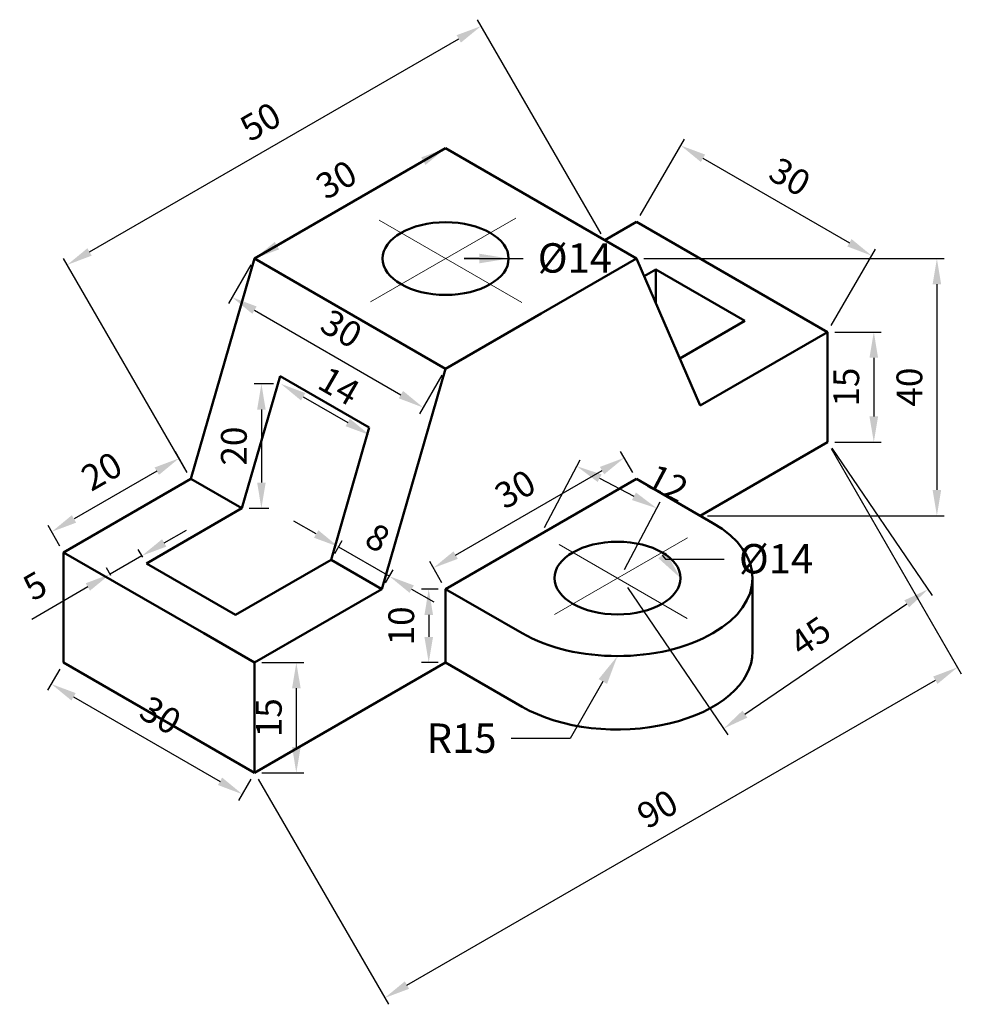
# Model space of a CAD drawing. Units: millimetres. Extents: x 3433 to 3561, y 1063 to 1197.
import ezdxf
from ezdxf import colors
from ezdxf.entities.mleader import LeaderData, LeaderLine
from ezdxf.math import Vec2, Vec3

# ---------------------------------------------------------------- set-up
doc = ezdxf.new("R2010")
doc.units = ezdxf.units.MM
doc.linetypes.add('CENTER', pattern=[50.8, 31.75, -6.35, 6.35, -6.35])
for name, color, linetype, lineweight in [('M-CNTR', 4, 'CENTER', 18), ('M-DIMS', 3, 'Continuous', 25), ('M-OUTL', 7, 'Continuous', 50), ('M-TEXT', 3, 'Continuous', 25)]:
    doc.layers.add(name, color=color, linetype=linetype, lineweight=lineweight)
doc.styles.get("Standard").update_dxf_attribs({"font": 'arial.ttf'})
doc.dimstyles.new('AM_ISO$0', dxfattribs={"dimtxt": 3.5, "dimasz": 3.5, "dimexe": 1, "dimexo": 1, "dimgap": 1.5, "dimtad": 1, "dimdsep": 46, "dimtxsty": 'Standard', "dimcen": 0, "dimclrd": 256, "dimclre": 256, "dimclrt": 2, "dimadec": 0, "dimazin": 2, "dimtp": 0.1, "dimtm": 0.1, "dimtfac": 0.71, "dimtdec": 3, "dimtmove": 0, "dimatfit": 3, "dimfxl": 1, "dimlwd": -1, "dimlwe": -1, "dimarcsym": 1})

# ---------------------------------------------------------------- blocks, each defined once
blk = doc.blocks.new('*D3')
at = {"layer": 'Defpoints', "color": 0, "transparency": 16777216}
for p in [(3542.53, 1154.98), (3542.53, 1139.98), (3548.82, 1139.98)]:
    blk.add_point(p, dxfattribs=at)
at = {"layer": 'M-DIMS', "color": 0, "linetype": 'ByBlock', "transparency": 16777216}
for p, q in [((3543.53, 1154.98), (3549.82, 1154.98)), ((3548.82, 1151.48), (3548.82, 1143.48)), ((3543.53, 1139.98), (3549.82, 1139.98))]:
    blk.add_line(p, q, dxfattribs=at)
at = {"layer": 'M-DIMS', "color": 0, "transparency": 16777216}
for points in [[(3548.23, 1151.48), (3549.4, 1151.48), (3548.82, 1154.98)], [(3548.23, 1143.48), (3549.4, 1143.48), (3548.82, 1139.98)]]:
    blk.add_solid(points, dxfattribs=at)
at = {"layer": 'M-DIMS', "color": 0, "transparency": 16777216, "insert": (3545.53, 1147.48), "char_height": 3.5, "attachment_point": 5, "rotation": 90}
blk.add_mtext('15', dxfattribs=at)
blk = doc.blocks.new('*D4')
at = {"layer": 'Defpoints', "color": 0, "transparency": 16777216}
for p in [(3516.55, 1169.98), (3548.53, 1165.37), (3542.53, 1154.98)]:
    blk.add_point(p, dxfattribs=at)
at = {"layer": 'M-DIMS', "color": 0, "linetype": 'ByBlock', "transparency": 16777216}
for p, q in [((3517.05, 1170.85), (3523.05, 1181.24)), ((3525.58, 1178.62), (3545.5, 1167.12)), ((3543.03, 1155.85), (3549.03, 1166.24))]:
    blk.add_line(p, q, dxfattribs=at)
at = {"layer": 'M-DIMS', "color": 0, "transparency": 16777216}
for points in [[(3525.87, 1179.13), (3525.29, 1178.12), (3522.55, 1180.37)], [(3545.79, 1167.63), (3545.21, 1166.62), (3548.53, 1165.37)]]:
    blk.add_solid(points, dxfattribs=at)
at = {"layer": 'M-DIMS', "color": 0, "transparency": 16777216, "insert": (3537.18, 1175.72), "char_height": 3.5, "attachment_point": 5, "rotation": 330}
blk.add_mtext('30', dxfattribs=at)
blk = doc.blocks.new('*D5')
at = {"layer": 'Defpoints', "color": 0, "transparency": 16777216}
for p in [(3449.87, 1123.48), (3444.93, 1122.03), (3445.53, 1120.98)]:
    blk.add_point(p, dxfattribs=at)
at = {"layer": 'M-DIMS', "color": 0, "linetype": 'ByBlock', "transparency": 16777216}
for p, q in [((3452.29, 1126.28), (3455.32, 1128.03)), ((3449.26, 1124.53), (3444.93, 1122.03)), ((3449.37, 1124.35), (3448.76, 1125.39)), ((3445.03, 1121.85), (3444.43, 1122.89)), ((3441.9, 1120.28), (3434.26, 1115.87))]:
    blk.add_line(p, q, dxfattribs=at)
at = {"layer": 'M-DIMS', "color": 0, "transparency": 16777216}
for points in [[(3452, 1126.78), (3452.58, 1125.77), (3449.26, 1124.53)], [(3441.61, 1120.78), (3442.19, 1119.77), (3444.93, 1122.03)]]:
    blk.add_solid(points, dxfattribs=at)
at = {"layer": 'M-DIMS', "color": 0, "transparency": 16777216, "insert": (3434.93, 1120.04), "char_height": 3.5, "attachment_point": 5, "rotation": 30}
blk.add_mtext('5', dxfattribs=at)
blk = doc.blocks.new('*D6')
at = {"layer": 'Defpoints', "color": 0, "transparency": 16777216}
for p in [(3455.93, 1134.98), (3436.99, 1127.79), (3438.61, 1124.98)]:
    blk.add_point(p, dxfattribs=at)
at = {"layer": 'M-DIMS', "color": 0, "linetype": 'ByBlock', "transparency": 16777216}
for p, q in [((3455.43, 1135.85), (3453.81, 1138.65)), ((3451.27, 1136.04), (3440.02, 1129.54)), ((3438.11, 1125.85), (3436.49, 1128.65))]:
    blk.add_line(p, q, dxfattribs=at)
at = {"layer": 'M-DIMS', "color": 0, "transparency": 16777216}
for points in [[(3450.98, 1136.54), (3451.57, 1135.53), (3454.31, 1137.79)], [(3439.72, 1130.04), (3440.31, 1129.03), (3436.99, 1127.79)]]:
    blk.add_solid(points, dxfattribs=at)
at = {"layer": 'M-DIMS', "color": 0, "transparency": 16777216, "insert": (3444, 1135.64), "char_height": 3.5, "attachment_point": 5, "rotation": 30}
blk.add_mtext('20', dxfattribs=at)
blk = doc.blocks.new('*D7')
at = {"layer": 'Defpoints', "color": 0, "transparency": 16777216}
for p in [(3490.57, 1179.98), (3464.59, 1164.98), (3464.59, 1164.98)]:
    blk.add_point(p, dxfattribs=at)
at = {"layer": 'M-DIMS', "color": 0, "linetype": 'ByBlock', "transparency": 16777216}
blk.add_line((3487.54, 1178.23), (3467.62, 1166.73), dxfattribs=at)
at = {"layer": 'M-DIMS', "color": 0, "transparency": 16777216}
for points in [[(3487.25, 1178.74), (3487.83, 1177.72), (3490.57, 1179.98)], [(3467.33, 1167.24), (3467.91, 1166.22), (3464.59, 1164.98)]]:
    blk.add_solid(points, dxfattribs=at)
at = {"layer": 'M-DIMS', "color": 0, "transparency": 16777216, "insert": (3475.93, 1175.33), "char_height": 3.5, "attachment_point": 5, "rotation": 30}
blk.add_mtext('30', dxfattribs=at)
blk = doc.blocks.new('*D8')
at = {"layer": 'Defpoints', "color": 0, "transparency": 16777216}
for p in [(3495.39, 1196.62), (3512.22, 1167.48), (3455.93, 1134.98)]:
    blk.add_point(p, dxfattribs=at)
at = {"layer": 'M-DIMS', "color": 0, "linetype": 'ByBlock', "transparency": 16777216}
for p, q in [((3511.72, 1168.35), (3494.89, 1197.49)), ((3442.13, 1165.87), (3492.36, 1194.87)), ((3455.43, 1135.85), (3438.6, 1164.99))]:
    blk.add_line(p, q, dxfattribs=at)
at = {"layer": 'M-DIMS', "color": 0, "transparency": 16777216}
for points in [[(3492.07, 1195.38), (3492.65, 1194.37), (3495.39, 1196.62)], [(3441.84, 1166.38), (3442.42, 1165.37), (3439.1, 1164.12)]]:
    blk.add_solid(points, dxfattribs=at)
at = {"layer": 'M-DIMS', "color": 0, "transparency": 16777216, "insert": (3465.6, 1183.22), "char_height": 3.5, "attachment_point": 5, "rotation": 30}
blk.add_mtext('50', dxfattribs=at)
blk = doc.blocks.new('*D9')
at = {"layer": 'Defpoints', "color": 0, "transparency": 16777216}
for p in [(3490.57, 1119.98), (3488.27, 1109.98), (3490.57, 1109.98)]:
    blk.add_point(p, dxfattribs=at)
at = {"layer": 'M-DIMS', "color": 0, "linetype": 'ByBlock', "transparency": 16777216}
for p, q in [((3489.57, 1119.98), (3487.27, 1119.98)), ((3488.27, 1116.48), (3488.27, 1113.48)), ((3489.57, 1109.98), (3487.27, 1109.98))]:
    blk.add_line(p, q, dxfattribs=at)
at = {"layer": 'M-DIMS', "color": 0, "transparency": 16777216}
for points in [[(3487.69, 1116.48), (3488.86, 1116.48), (3488.27, 1119.98)], [(3487.69, 1113.48), (3488.86, 1113.48), (3488.27, 1109.98)]]:
    blk.add_solid(points, dxfattribs=at)
at = {"layer": 'M-DIMS', "color": 0, "transparency": 16777216, "insert": (3484.99, 1114.98), "char_height": 3.5, "attachment_point": 5, "rotation": 90}
blk.add_mtext('10', dxfattribs=at)
blk = doc.blocks.new('*D10')
at = {"layer": 'Defpoints', "color": 0, "transparency": 16777216}
for p in [(3514.88, 1137.86), (3516.55, 1134.98), (3490.57, 1119.98)]:
    blk.add_point(p, dxfattribs=at)
at = {"layer": 'M-DIMS', "color": 0, "linetype": 'ByBlock', "transparency": 16777216}
for p, q in [((3516.05, 1135.85), (3514.38, 1138.73)), ((3491.93, 1124.61), (3511.85, 1136.11)), ((3490.07, 1120.85), (3488.4, 1123.73))]:
    blk.add_line(p, q, dxfattribs=at)
at = {"layer": 'M-DIMS', "color": 0, "transparency": 16777216}
for points in [[(3511.56, 1136.62), (3512.14, 1135.61), (3514.88, 1137.86)], [(3491.64, 1125.12), (3492.23, 1124.11), (3488.9, 1122.86)]]:
    blk.add_solid(points, dxfattribs=at)
at = {"layer": 'M-DIMS', "color": 0, "transparency": 16777216, "insert": (3500.25, 1133.21), "char_height": 3.5, "attachment_point": 5, "rotation": 30}
blk.add_mtext('30', dxfattribs=at)
blk = doc.blocks.new('*D11')
at = {"layer": 'Defpoints', "color": 0, "transparency": 16777216}
for p in [(3519.29, 1130.99), (3503.56, 1127.48), (3514.43, 1121.76)]:
    blk.add_point(p, dxfattribs=at)
at = {"layer": 'M-DIMS', "color": 0, "linetype": 'ByBlock', "transparency": 16777216}
for p, q in [((3504.02, 1128.36), (3508.89, 1137.6)), ((3511.52, 1135.08), (3516.19, 1132.62)), ((3514.89, 1122.64), (3519.76, 1131.87))]:
    blk.add_line(p, q, dxfattribs=at)
at = {"layer": 'M-DIMS', "color": 0, "transparency": 16777216}
for points in [[(3511.79, 1135.6), (3511.25, 1134.56), (3508.42, 1136.71)], [(3516.46, 1133.13), (3515.92, 1132.1), (3519.29, 1130.99)]]:
    blk.add_solid(points, dxfattribs=at)
at = {"layer": 'M-DIMS', "color": 0, "transparency": 16777216, "insert": (3520.56, 1134), "char_height": 3.5, "attachment_point": 5, "rotation": 332.2232}
blk.add_mtext('12', dxfattribs=at)
blk = doc.blocks.new('*D12')
at = {"layer": 'Defpoints', "color": 0, "transparency": 16777216}
for p in [(3464.59, 1109.98), (3464.59, 1094.98), (3470.26, 1094.98)]:
    blk.add_point(p, dxfattribs=at)
at = {"layer": 'M-DIMS', "color": 0, "linetype": 'ByBlock', "transparency": 16777216}
for p, q in [((3465.59, 1109.98), (3471.26, 1109.98)), ((3470.26, 1106.48), (3470.26, 1098.48)), ((3465.59, 1094.98), (3471.26, 1094.98))]:
    blk.add_line(p, q, dxfattribs=at)
at = {"layer": 'M-DIMS', "color": 0, "transparency": 16777216}
for points in [[(3469.68, 1106.48), (3470.85, 1106.48), (3470.26, 1109.98)], [(3469.68, 1098.48), (3470.85, 1098.48), (3470.26, 1094.98)]]:
    blk.add_solid(points, dxfattribs=at)
at = {"layer": 'M-DIMS', "color": 0, "transparency": 16777216, "insert": (3466.98, 1102.48), "char_height": 3.5, "attachment_point": 5, "rotation": 90}
blk.add_mtext('15', dxfattribs=at)
blk = doc.blocks.new('*D13')
at = {"layer": 'Defpoints', "color": 0, "transparency": 16777216}
for p in [(3438.61, 1109.98), (3464.59, 1094.98), (3462.91, 1092.07)]:
    blk.add_point(p, dxfattribs=at)
at = {"layer": 'M-DIMS', "color": 0, "linetype": 'ByBlock', "transparency": 16777216}
for p, q in [((3438.11, 1109.11), (3436.43, 1106.21)), ((3439.96, 1105.32), (3459.88, 1093.82)), ((3464.09, 1094.11), (3462.41, 1091.21))]:
    blk.add_line(p, q, dxfattribs=at)
at = {"layer": 'M-DIMS', "color": 0, "transparency": 16777216}
for points in [[(3440.25, 1105.83), (3439.67, 1104.82), (3436.93, 1107.07)], [(3460.17, 1094.33), (3459.59, 1093.32), (3462.91, 1092.07)]]:
    blk.add_solid(points, dxfattribs=at)
at = {"layer": 'M-DIMS', "color": 0, "transparency": 16777216, "insert": (3451.56, 1102.42), "char_height": 3.5, "attachment_point": 5, "rotation": 330}
blk.add_mtext('30', dxfattribs=at)
blk = doc.blocks.new('*D14')
at = {"layer": 'Defpoints', "color": 0, "transparency": 16777216}
for p in [(3468.16, 1147.92), (3480.29, 1140.92), (3480.29, 1140.92)]:
    blk.add_point(p, dxfattribs=at)
at = {"layer": 'M-DIMS', "color": 0, "linetype": 'ByBlock', "transparency": 16777216}
blk.add_line((3471.19, 1146.17), (3477.25, 1142.67), dxfattribs=at)
at = {"layer": 'M-DIMS', "color": 0, "transparency": 16777216}
for points in [[(3471.48, 1146.67), (3470.9, 1145.66), (3468.16, 1147.92)], [(3477.55, 1143.17), (3476.96, 1142.16), (3480.29, 1140.92)]]:
    blk.add_solid(points, dxfattribs=at)
at = {"layer": 'M-DIMS', "color": 0, "transparency": 16777216, "insert": (3475.85, 1147.24), "char_height": 3.5, "attachment_point": 5, "rotation": 330}
blk.add_mtext('14', dxfattribs=at)
blk = doc.blocks.new('*D15')
at = {"layer": 'Defpoints', "color": 0, "transparency": 16777216}
for p in [(3474.98, 1123.98), (3482.92, 1121.74), (3481.91, 1119.98)]:
    blk.add_point(p, dxfattribs=at)
at = {"layer": 'M-DIMS', "color": 0, "linetype": 'ByBlock', "transparency": 16777216}
for p, q in [((3472.96, 1127.49), (3469.93, 1129.24)), ((3475.48, 1124.85), (3476.49, 1126.6)), ((3475.99, 1125.74), (3482.92, 1121.74)), ((3482.41, 1120.85), (3483.42, 1122.6)), ((3485.95, 1119.99), (3488.98, 1118.24))]:
    blk.add_line(p, q, dxfattribs=at)
at = {"layer": 'M-DIMS', "color": 0, "transparency": 16777216}
for points in [[(3473.26, 1127.99), (3472.67, 1126.98), (3475.99, 1125.74)], [(3486.25, 1120.49), (3485.66, 1119.48), (3482.92, 1121.74)]]:
    blk.add_solid(points, dxfattribs=at)
at = {"layer": 'M-DIMS', "color": 0, "transparency": 16777216, "insert": (3481.1, 1126.58), "char_height": 3.5, "attachment_point": 5, "rotation": 330}
blk.add_mtext('8', dxfattribs=at)
blk = doc.blocks.new('*D16')
at = {"layer": 'Defpoints', "color": 0, "transparency": 16777216}
for p in [(3464.59, 1164.98), (3490.57, 1149.98), (3487.52, 1144.7)]:
    blk.add_point(p, dxfattribs=at)
at = {"layer": 'M-DIMS', "color": 0, "linetype": 'ByBlock', "transparency": 16777216}
for p, q in [((3464.09, 1164.11), (3461.04, 1158.84)), ((3464.57, 1157.95), (3484.49, 1146.45)), ((3490.07, 1149.11), (3487.02, 1143.84))]:
    blk.add_line(p, q, dxfattribs=at)
at = {"layer": 'M-DIMS', "color": 0, "transparency": 16777216}
for points in [[(3464.86, 1158.46), (3464.28, 1157.45), (3461.54, 1159.7)], [(3484.78, 1146.96), (3484.2, 1145.95), (3487.52, 1144.7)]]:
    blk.add_solid(points, dxfattribs=at)
at = {"layer": 'M-DIMS', "color": 0, "transparency": 16777216, "insert": (3476.18, 1155.05), "char_height": 3.5, "attachment_point": 5, "rotation": 330}
blk.add_mtext('30', dxfattribs=at)
blk = doc.blocks.new('*D17')
at = {"layer": 'Defpoints', "color": 0, "transparency": 16777216}
for p in [(3542.53, 1139.98), (3560.22, 1109.34), (3464.59, 1094.98)]:
    blk.add_point(p, dxfattribs=at)
at = {"layer": 'M-DIMS', "color": 0, "linetype": 'ByBlock', "transparency": 16777216}
for p, q in [((3543.03, 1139.11), (3560.72, 1108.47)), ((3485.31, 1066.09), (3557.19, 1107.59)), ((3465.09, 1094.11), (3482.78, 1063.47))]:
    blk.add_line(p, q, dxfattribs=at)
at = {"layer": 'M-DIMS', "color": 0, "transparency": 16777216}
for points in [[(3556.9, 1108.09), (3557.48, 1107.08), (3560.22, 1109.34)], [(3485.02, 1066.59), (3485.6, 1065.58), (3482.28, 1064.34)]]:
    blk.add_solid(points, dxfattribs=at)
at = {"layer": 'M-DIMS', "color": 0, "transparency": 16777216, "insert": (3519.61, 1089.68), "char_height": 3.5, "attachment_point": 5, "rotation": 30}
blk.add_mtext('90', dxfattribs=at)
blk = doc.blocks.new('*D18')
at = {"layer": 'Defpoints', "color": 0, "transparency": 16777216}
for p in [(3542.53, 1139.98), (3514.74, 1121.03), (3556.19, 1119.95)]:
    blk.add_point(p, dxfattribs=at)
at = {"layer": 'M-DIMS', "color": 0, "linetype": 'ByBlock', "transparency": 16777216}
for p, q in [((3543.09, 1139.15), (3556.75, 1119.13)), ((3515.3, 1120.2), (3528.96, 1100.17)), ((3531.29, 1102.97), (3553.3, 1117.98))]:
    blk.add_line(p, q, dxfattribs=at)
at = {"layer": 'M-DIMS', "color": 0, "transparency": 16777216}
for points in [[(3552.97, 1118.46), (3553.62, 1117.5), (3556.19, 1119.95)], [(3530.96, 1103.45), (3531.61, 1102.49), (3528.39, 1101)]]:
    blk.add_solid(points, dxfattribs=at)
at = {"layer": 'M-DIMS', "color": 0, "transparency": 16777216, "insert": (3540.44, 1113.19), "char_height": 3.5, "attachment_point": 5, "rotation": 34.2921}
blk.add_mtext('45', dxfattribs=at)
blk = doc.blocks.new('*D19')
at = {"layer": 'Defpoints', "color": 0, "transparency": 16777216}
for p in [(3468.16, 1147.92), (3462.86, 1130.98), (3465.51, 1130.98)]:
    blk.add_point(p, dxfattribs=at)
at = {"layer": 'M-DIMS', "color": 0, "linetype": 'ByBlock', "transparency": 16777216}
for p, q in [((3467.16, 1147.92), (3464.51, 1147.92)), ((3465.51, 1144.42), (3465.51, 1134.48)), ((3463.86, 1130.98), (3466.51, 1130.98))]:
    blk.add_line(p, q, dxfattribs=at)
at = {"layer": 'M-DIMS', "color": 0, "transparency": 16777216}
for points in [[(3464.93, 1144.42), (3466.09, 1144.42), (3465.51, 1147.92)], [(3464.93, 1134.48), (3466.09, 1134.48), (3465.51, 1130.98)]]:
    blk.add_solid(points, dxfattribs=at)
at = {"layer": 'M-DIMS', "color": 0, "transparency": 16777216, "insert": (3462.22, 1139.45), "char_height": 3.5, "attachment_point": 5, "rotation": 90}
blk.add_mtext('20', dxfattribs=at)
blk = doc.blocks.new('*D20')
at = {"layer": 'Defpoints', "color": 0, "transparency": 16777216}
for p in [(3516.55, 1164.98), (3525.21, 1129.98), (3557.4, 1129.98)]:
    blk.add_point(p, dxfattribs=at)
at = {"layer": 'M-DIMS', "color": 0, "linetype": 'ByBlock', "transparency": 16777216}
for p, q in [((3517.55, 1164.98), (3558.4, 1164.98)), ((3557.4, 1161.48), (3557.4, 1133.48)), ((3526.21, 1129.98), (3558.4, 1129.98))]:
    blk.add_line(p, q, dxfattribs=at)
at = {"layer": 'M-DIMS', "color": 0, "transparency": 16777216}
for points in [[(3556.82, 1161.48), (3557.98, 1161.48), (3557.4, 1164.98)], [(3556.82, 1133.48), (3557.98, 1133.48), (3557.4, 1129.98)]]:
    blk.add_solid(points, dxfattribs=at)
at = {"layer": 'M-DIMS', "color": 0, "transparency": 16777216, "insert": (3554.11, 1147.48), "char_height": 3.5, "attachment_point": 5, "rotation": 90}
blk.add_mtext('40', dxfattribs=at)

msp = doc.modelspace()

# ---------------------------------------------------------------- linework, layer by layer
at = {"layer": 'M-CNTR'}
for p, q in [((3500.11, 1170.489), (3480.337, 1159.073)), ((3481.534, 1170.196), (3500.942, 1158.991)), ((3523.477, 1126.98), (3505.378, 1116.53)), ((3523.446, 1115.998), (3506.027, 1126.055))]:
    msp.add_line(p, q, dxfattribs=at)
at = {"layer": 'M-OUTL'}
for p, q in [((3464.587, 1164.98), (3490.568, 1179.98)), ((3490.568, 1179.98), (3516.549, 1164.98)), ((3512.219, 1167.48), (3516.549, 1169.98)), ((3542.53, 1154.98), (3516.549, 1169.98)), ((3455.927, 1134.98), (3464.587, 1164.98)), ((3490.568, 1149.98), (3464.587, 1164.98)), ((3516.549, 1164.98), (3503.559, 1157.48)), ((3525.209, 1144.98), (3516.549, 1164.98)), ((3517.588, 1162.58), (3519.147, 1163.48)), ((3519.147, 1163.48), (3531.271, 1156.48)), ((3519.147, 1158.98), (3519.147, 1163.48)), ((3503.559, 1157.48), (3490.568, 1149.98)), ((3531.271, 1156.48), (3522.438, 1151.38)), ((3525.209, 1144.98), (3542.53, 1154.98)), ((3542.53, 1139.98), (3542.53, 1154.98)), ((3481.908, 1119.98), (3490.568, 1149.98)), ((3468.052, 1148.98), (3462.855, 1130.98)), ((3480.176, 1141.98), (3468.052, 1148.98)), ((3480.176, 1141.98), (3474.98, 1123.98)), ((3542.53, 1139.98), (3525.209, 1129.98)), ((3525.209, 1129.98), (3542.53, 1139.98)), ((3438.607, 1124.98), (3455.927, 1134.98)), ((3455.927, 1134.98), (3462.855, 1130.98)), ((3490.568, 1119.98), (3516.549, 1134.98)), ((3526.941, 1128.98), (3516.549, 1134.98)), ((3462.855, 1130.98), (3449.865, 1123.48)), ((3462.855, 1130.98), (3449.865, 1123.48)), ((3449.865, 1123.48), (3462.855, 1130.98)), ((3438.607, 1109.98), (3438.607, 1124.98)), ((3438.607, 1124.98), (3445.535, 1120.98)), ((3449.865, 1123.48), (3461.989, 1116.48)), ((3474.98, 1123.98), (3461.989, 1116.48)), ((3481.908, 1119.98), (3474.98, 1123.98)), ((3445.535, 1120.98), (3457.659, 1113.98)), ((3532.322, 1111.48), (3532.322, 1121.48)), ((3464.587, 1109.98), (3481.908, 1119.98)), ((3500.961, 1113.98), (3490.568, 1119.98)), ((3490.568, 1119.98), (3490.568, 1109.98)), ((3457.659, 1113.98), (3464.587, 1109.98)), ((3438.607, 1109.98), (3464.587, 1094.98)), ((3464.587, 1094.98), (3490.568, 1109.98)), ((3464.587, 1094.98), (3464.587, 1109.98)), ((3464.587, 1094.98), (3490.568, 1109.98)), ((3500.961, 1103.98), (3490.568, 1109.98))]:
    msp.add_line(p, q, dxfattribs=at)
for centre in [(3490.568, 1164.98), (3513.951, 1121.48)]:
    msp.add_ellipse(centre, major_axis=(-8.573, 0), ratio=0.5773503, dxfattribs=at)
for centre, end_param in [((3513.951, 1121.48), 3.9269908), ((3513.951, 1111.48), 3.1415927)]:
    msp.add_ellipse(centre, major_axis=(-18.371, 0), ratio=0.5773503, start_param=0.7853982, end_param=end_param, dxfattribs=at)

# ---------------------------------------------------------------- dimensions: what is measured, and where the dimension line sits
at = {"layer": 'M-DIMS'}
for p1, p2, distance, text, picture, middle in [((3455.927, 1134.98), (3512.219, 1167.48), 33.651, '50', '*D8', (3465.604, 1183.219)), ((3514.737, 1121.027), (3542.53, 1139.98), -24.24, '45', '*D18', (3540.443, 1113.186))]:
    dim = msp.add_aligned_dim(p1=p1, p2=p2, distance=distance, text=text, dimstyle='AM_ISO$0', override={"dimpost": '', "dimclrd": 0, "dimclre": 0, "dimclrt": 0}, dxfattribs=at)
    dim.commit()
    dim.dimension.update_dxf_attribs({"geometry": picture, "text_midpoint": middle})
for p1, p2, distance, override, picture, middle in [((3516.549, 1169.98), (3542.53, 1154.98), 12, {"dimclrd": 0, "dimclre": 0, "dimclrt": 0}, '*D4', (3537.183, 1175.72)), ((3490.568, 1179.98), (3464.587, 1164.98), 0, {"dimclrd": 0, "dimclre": 0, "dimclrt": 0}, '*D7', (3475.934, 1175.328)), ((3468.161, 1147.917), (3480.286, 1140.917), 0, {"dimclrd": 0, "dimclre": 0, "dimclrt": 0}, '*D14', (3475.852, 1147.238)), ((3464.587, 1094.98), (3542.53, 1139.98), -35.383, {"dimclrd": 0, "dimclre": 0, "dimclrt": 0}, '*D17', (3519.606, 1089.684)), ((3455.927, 1134.98), (3438.607, 1124.98), -3.243, {"dimclrd": 0, "dimclre": 0, "dimclrt": 0}, '*D6', (3444.002, 1135.636)), ((3490.568, 1119.98), (3516.549, 1134.98), 3.331, {"dimclrd": 0, "dimclre": 0, "dimclrt": 0}, '*D10', (3500.249, 1133.212)), ((3474.98, 1123.98), (3481.908, 1119.98), 2.029, {"dimclrd": 0, "dimclre": 0, "dimclrt": 0}, '*D15', (3481.102, 1126.584)), ((3449.865, 1123.48), (3445.535, 1120.98), -1.207, {"dimclrd": 0, "dimclre": 0, "dimclrt": 0}, '*D5', (3434.925, 1120.036)), ((3490.568, 1119.98), (3490.568, 1109.98), -2.294, {"dimpost": '', "dimclrd": 0, "dimclre": 0, "dimclrt": 0}, '*D9', (3484.987, 1114.98)), ((3438.607, 1109.98), (3464.587, 1094.98), -3.358, {"dimclrd": 0, "dimclre": 0, "dimclrt": 0}, '*D13', (3451.562, 1102.42))]:
    dim = msp.add_aligned_dim(p1=p1, p2=p2, distance=distance, dimstyle='AM_ISO$0', override=override, dxfattribs=at)
    dim.commit()
    dim.dimension.update_dxf_attribs({"geometry": picture, "text_midpoint": middle})
for base, p1, p2, angle, picture, middle in [((3487.522, 1144.704), (3464.587, 1164.98), (3490.568, 1149.98), 330, '*D16', (3474.532, 1152.204)), ((3548.817, 1139.98), (3542.53, 1154.98), (3542.53, 1139.98), 270, '*D3', (3548.817, 1147.48)), ((3470.263, 1094.98), (3464.587, 1109.98), (3464.587, 1094.98), 270, '*D12', (3470.263, 1102.48))]:
    dim = msp.add_linear_dim(base=base, p1=p1, p2=p2, angle=angle, dimstyle='AM_ISO$0', override={"dimclrd": 0, "dimclre": 0, "dimclrt": 0}, dxfattribs=at)
    dim.commit()
    dim.dimension.update_dxf_attribs({"geometry": picture, "text_midpoint": middle, "dimtype": 161})
dim = msp.add_linear_dim(base=(3557.4, 1129.98), p1=(3516.549, 1164.98), p2=(3525.209, 1129.98), angle=90, text='40', dimstyle='AM_ISO$0', override={"dimpost": '', "dimclrd": 0, "dimclre": 0, "dimclrt": 0}, dxfattribs=at)
dim.commit()
dim.dimension.update_dxf_attribs({"geometry": '*D20', "text_midpoint": (3554.113, 1147.48)})
for base, p1, p2, angle, text, picture, middle, dimtype in [((3465.508, 1130.98), (3468.161, 1147.917), (3462.855, 1130.98), 90, '20', '*D19', (3465.508, 1139.448), 160), ((3519.29, 1130.986), (3503.559, 1127.48), (3514.427, 1121.755), 332.22316, '12', '*D11', (3519.044, 1131.116), 161)]:
    dim = msp.add_linear_dim(base=base, p1=p1, p2=p2, angle=angle, text=text, dimstyle='AM_ISO$0', override={"dimclrd": 0, "dimclre": 0, "dimclrt": 0}, dxfattribs=at)
    dim.commit()
    dim.dimension.update_dxf_attribs({"geometry": picture, "text_midpoint": middle, "dimtype": dimtype})

# ---------------------------------------------------------------- leaders
at = {"layer": 'M-TEXT'}
ml = msp.add_multileader_mtext('Standard', dxfattribs=at)
ml.set_content('{\\C2;%%C14}', color=256)
ml.set_leader_properties()
ml.build(insert=Vec2(0, 0))
ctx = ml.context
ctx.base_point, ctx.plane_origin = Vec3(3501.106, 1164.98), Vec3(3499.141, 1164.98)
notes = []
notes.append((ctx, [(0, (1, 1, 0), (3493.106, 1164.98), (1, 0), 8, [(0, [(3499.141, 1164.98)], 0, [])])]))
ctx.mtext.insert, ctx.mtext.flow_direction = Vec3(3503.106, 1167.061), 5
ml = msp.add_multileader_mtext('Standard', dxfattribs=at)
ml.set_content('{\\C2;%%C14}', color=256)
ml.set_leader_properties()
ml.build(insert=Vec2(0, 0))
ctx = ml.context
ctx.base_point, ctx.plane_origin = Vec3(3528.471, 1124.039), Vec3(3522.524, 1121.48)
notes.append((ctx, [(1, (1, 1, 0), (3520.471, 1124.039), (1, 0), 8, [(0, [(3522.524, 1121.48)], 0, [])])]))
ctx.mtext.insert, ctx.mtext.flow_direction = Vec3(3530.471, 1126.12), 5
ml = msp.add_multileader_mtext('Standard', dxfattribs=at)
ml.set_content('{\\C2;R15}', color=256)
ml.set_leader_properties()
ml.build(insert=Vec2(0, 0))
ctx = ml.context
ctx.base_point, ctx.plane_origin = Vec3(3485.913, 1099.66), Vec3(3513.951, 1110.874)
ctx.text_align_type = 2
notes.append((ctx, [(0, (1, 1, 0), (3507.501, 1099.66), (-1, 0), 8, [(0, [(3513.951, 1110.874)], 0, [])])]))
ctx.mtext.insert, ctx.mtext.alignment, ctx.mtext.flow_direction = Vec3(3497.501, 1101.694), 3, 5
for ctx, leaders in notes:
    for number, flags, end, landing, length, lines in leaders:
        leader = LeaderData()
        leader.index, (leader.has_last_leader_line, leader.has_dogleg_vector, leader.attachment_direction) = number, flags
        leader.last_leader_point, leader.dogleg_vector, leader.dogleg_length = Vec3(end), Vec3(landing), length
        for number, points, colour, breaks in lines:
            line = LeaderLine()
            line.index, line.vertices, line.color, line.breaks = number, Vec3.list(points), colors.encode_raw_color(colour), breaks
            leader.lines.append(line)
        ctx.leaders.append(leader)

doc.saveas('drawing.dxf')
